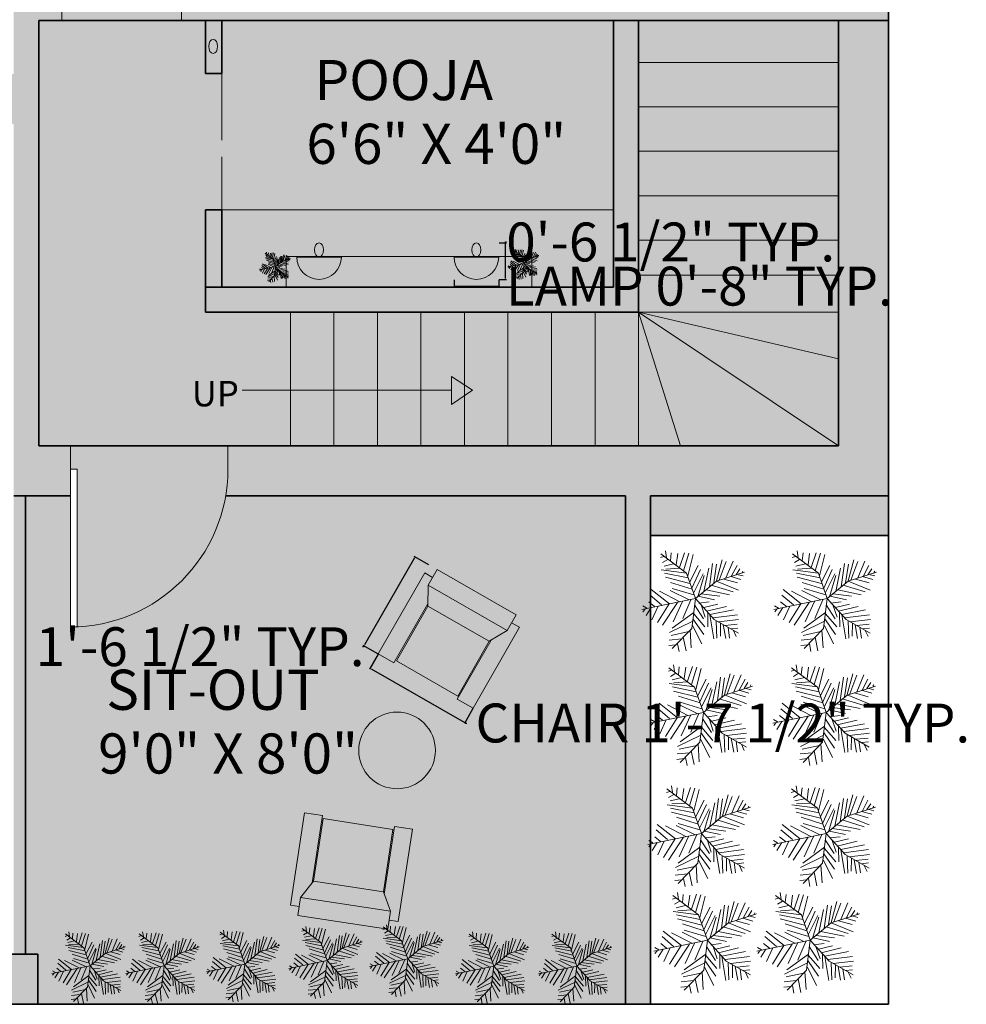
# Model space of a CAD drawing. Units: inches. Extents: x 2167 to 2589, y 1680 to 2489.
# Tile 30 of 38: x 2419 to 2589, y 1688 to 1865. Entities that reach past the tile are written whole.
import ezdxf

# ---------------------------------------------------------------- set-up
doc = ezdxf.new("R2010")
doc.units = ezdxf.units.IN
doc.header["$MEASUREMENT"] = 0
doc.linetypes.add('ACAD_ISO02W100', pattern=[15, 12, -3])
doc.layers.get('0').update_dxf_attribs({"color": 250})
for name, color, linetype, lineweight in [('A-ANNO-DIMS', 2, 'Continuous', 18), ('A-ANNO-SYMB', 7, 'Continuous', 18), ('A-AREA-IDEN', 7, 'Continuous', 18), ('A-DOOR', 4, 'Continuous', 18), ('A-FLOR-STRS', 7, 'Continuous', 18), ('A-FURN-FIXD', 34, 'Continuous', 18), ('A-FURN-PATT', 31, 'Continuous', 13), ('A-WALL-OVHD', 8, 'ACAD_ISO02W100', 18), ('A-WALL-PATT', 250, 'Continuous', 13), ('C-PROP', 7, 'Continuous', 35), ('furniture', 34, 'Continuous', 18), ('L-PLNT', 106, 'Continuous', 13), ('L-PVMT-PATT', 252, 'Continuous', 13), ('walls', 7, 'Continuous', 35)]:
    doc.layers.add(name, color=color, linetype=linetype, lineweight=lineweight)
for name, color, linetype, lineweight, true_color in [('A-FLOR-PATT', 254, 'Continuous', 13, 0xfeeab9), ('A-FLOR-STRS-PATT', 33, 'Continuous', 13, 0xcda06d), ('A-FURN-FIXD-PATT', 33, 'Continuous', 13, 0xcd8e5c)]:
    doc.layers.add(name, color=color, linetype=linetype, lineweight=lineweight, true_color=true_color)
doc.styles.get("Standard").update_dxf_attribs({"font": 'arial.ttf'})
doc.dimstyles.get("Standard").update_dxf_attribs({"dimtxt": 7, "dimasz": 0.18, "dimexe": 0.18, "dimexo": 0.0625, "dimgap": 0.09, "dimtad": 0, "dimtih": 1, "dimtoh": 1, "dimdec": 1, "dimzin": 0, "dimdsep": 46, "dimlunit": 3, "dimtxsty": 'Standard', "dimcen": 0.09, "dimadec": 0, "dimazin": 0, "dimtfac": 1, "dimtdec": 1, "dimtofl": 0, "dimtmove": 0, "dimatfit": 3, "dimfxl": 1, "dimtolj": 1, "dimtzin": 0, "dimarcsym": 0})

# ---------------------------------------------------------------- blocks, each defined once
blk = doc.blocks.new('*U2')
for p, q in [((0, 0), (0, -6)), ((40, 0), (40, -6))]:
    blk.add_line(p, q)
blk.add_lwpolyline([(0, 0), (0, 40), (1.75, 40), (1.75, 0)], close=True)
blk.add_arc((0, 0), 40, 0, 90)
blk = doc.blocks.new('*U8')
for p, q in [((-8.737, 47.138), (-17.069, 52.711)), ((-10.186, 53.64), (-13.084, 55.962)), ((0, 0), (-10.5, 57)), ((-9.099, 51.782), (-6.563, 55.962)), ((-7.288, 39.707), (-21.778, 46.673)), ((-7.65, 43.423), (-2.578, 49.46)), ((-5.839, 35.992), (4.667, 48.067)), ((-5.114, 27.632), (10.463, 46.673)), ((-3.665, 19.273), (-27.574, 35.527)), ((-5.114, 28.097), (-24.676, 40.636)), ((-2.941, 16.486), (8.652, 37.85)), ((16.259, 5.805), (23.142, 31.348)), ((22.055, 7.198), (27.489, 32.277)), ((27, 9), (48, 36)), ((27.127, 9.056), (31.112, 35.992)), ((35.096, 32.741), (37.27, 22.524)), ((38.719, 34.134), (41.979, 28.561)), ((44.153, 36.456), (45.239, 32.741)), ((-31.5, 4.5), (-52.5, 25.5)), ((-48.585, 21.131), (-49.309, 29.026)), ((-43.513, 28.561), (-42.427, 15.558)), ((-38.442, 26.239), (-34.819, 7.663)), ((-35.544, 28.097), (-24.314, 3.947)), ((-14.533, 2.09), (-30.834, 25.31)), ((-24.314, 23.917), (-2.941, 13.7)), ((-1.129, 6.734), (9.014, 26.704)), ((3.942, 1.625), (11.187, 24.381)), ((10.101, 3.483), (17.708, 26.239)), ((31.836, 30.883), (32.561, 16.486)), ((40.53, 25.775), (48.862, 24.846)), ((43.791, 29.954), (51.036, 30.883)), ((-47.498, 19.737), (-55.83, 18.344)), ((-40.615, 13.7), (-55.105, 10.913)), ((-20.691, 13.7), (-1.129, 4.876)), ((29.662, 12.307), (48.137, 6.269)), ((33.285, 16.486), (48.862, 10.913)), ((36.183, 19.737), (48.137, 17.88)), ((-33.37, 6.269), (-52.207, 5.34)), ((-28.299, 3.483), (-47.86, -5.805)), ((-21.416, 3.018), (-38.079, -8.128)), ((0, 0), (-31.5, 4.5)), ((-15.982, 2.09), (-30.11, -9.521)), ((0, 0), (-22.5, -19.5)), ((-6.563, 1.161), (-21.416, -8.128)), ((0, 0), (27, 9)), ((0, 0), (18, -22.5)), ((6.478, 1.625), (26.04, -8.592)), ((11.187, 3.483), (30.749, -5.805)), ((18.07, 5.805), (35.096, -3.483)), ((24.229, 7.663), (46.688, 1.625)), ((-6.563, -5.805), (-19.967, -9.985)), ((-9.461, -8.592), (-6.201, -23.453)), ((-4.752, -3.483), (-3.665, -14.629)), ((2.493, -3.019), (-1.491, -20.202)), ((1.769, -2.555), (24.229, -9.521)), ((5.029, -6.27), (2.131, -25.775)), ((7.565, -9.056), (32.198, -14.629)), ((-17.431, -15.094), (-42.789, -18.809)), ((-22.5, -19.5), (-37.5, -45)), ((-15.257, -12.772), (-30.11, -12.772)), ((-20.691, -18.345), (-17.793, -44.352)), ((-17.069, -15.094), (-12.721, -40.172)), ((-13.446, -11.378), (-8.737, -32.741)), ((9.014, -11.378), (3.58, -35.992)), ((14.085, -16.951), (6.478, -40.172)), ((12.274, -15.094), (36.907, -18.809)), ((16.259, -19.738), (36.183, -22.989)), ((-28.299, -29.026), (-42.789, -31.348)), ((-24.314, -21.596), (-42.427, -22.06)), ((-26.849, -26.24), (-40.253, -25.775)), ((-29.023, -30.884), (-27.936, -43.887)), ((-25.038, -23.918), (-22.865, -45.281)), ((18.07, -22.524), (8.289, -45.745)), ((20.244, -30.419), (15.897, -44.816)), ((18, -22.5), (27, -52.5)), ((18.433, -22.524), (40.53, -29.026)), ((19.157, -25.311), (38.719, -33.206)), ((-30.834, -34.135), (-42.427, -35.528)), ((-34.457, -39.708), (-40.978, -42.494)), ((-32.646, -36.921), (-31.921, -44.352)), ((22.78, -37.85), (19.519, -48.532)), ((21.331, -32.741), (39.081, -40.636)), ((22.78, -38.314), (34.372, -44.816)), ((24.591, -45.745), (23.142, -50.854)), ((24.591, -43.423), (30.749, -47.603)), ((26.764, -49.925), (28.213, -50.854))]:
    blk.add_line(p, q)
blk = doc.blocks.new('FABRIC SOFA 1S')
at = {"layer": 'furniture'}
for p, q in [((3, 18.12), (34, 18.12)), ((3, 15.12), (3, 18.12)), ((34, 12.12), (34, 18.12)), ((0, -15.12), (0, 15.12)), ((6, 15.12), (0, 15.12)), ((6, -15.12), (6, 15.12)), ((12, 11.75), (6, 15.12)), ((11.33, 12.12), (34, 12.12)), ((6, -15.12), (12, -11.75)), ((11.33, -12.12), (34, -12.12)), ((34, -12.12), (34, -18.12)), ((6, -15.12), (0, -15.12)), ((3, -18.12), (3, -15.12)), ((3, -18.12), (34, -18.12))]:
    blk.add_line(p, q, dxfattribs=at)
blk.add_lwpolyline([(12, -11.75), (12, 11.75), (33, 11.75), (33, -11.75)], close=True, dxfattribs=at)
blk = doc.blocks.new('POOJA-LAMP')
h = blk.add_hatch(color=256)
h.dxf.hatch_style = 1
edge = h.paths.add_edge_path()
edge.add_ellipse((4.02, 5.29), major_axis=(0, -1.27), ratio=0.637064, start_angle=0, end_angle=360)
blk.add_line((0, 4.02), (8.04, 4.02))
blk.add_arc((4.02, 4.02), 4.02, 180, 0)
blk.add_ellipse((4.02, 5.29), major_axis=(0, -1.27), ratio=0.637064)
blk = doc.blocks.new('*D29')
at = {"layer": 'A-ANNO-DIMS', "color": 0, "lineweight": -2, "transparency": 16777216}
for p, q in [((2483.15, 1750.65), (2481.62, 1747.99)), ((2481.87, 1748.06), (2498.61, 1738.47)), ((2500.2, 1740.88), (2498.67, 1738.22)), ((2498.76, 1738.38), (2498.92, 1738.29)), ((2498.92, 1738.29), (2499.1, 1738.29))]:
    blk.add_line(p, q, dxfattribs=at)
at = {"layer": 'A-ANNO-DIMS', "color": 0, "transparency": 16777216}
for points in [[(2481.88, 1748.09), (2481.85, 1748.04), (2481.71, 1748.15)], [(2498.62, 1738.5), (2498.59, 1738.44), (2498.76, 1738.38)]]:
    blk.add_solid(points, dxfattribs=at)
at = {"layer": 'Defpoints', "color": 0, "transparency": 16777216}
for p in [(2483.18, 1750.71), (2500.23, 1740.94), (2498.76, 1738.38)]:
    blk.add_point(p, dxfattribs=at)
at = {"layer": 'A-ANNO-DIMS', "color": 0, "transparency": 16777216, "insert": (2545.21, 1738.29), "char_height": 7, "attachment_point": 5}
blk.add_mtext('\\A1;CHAIR 1\'-7 1/2" TYP.', dxfattribs=at)
blk = doc.blocks.new('*D30')
at = {"layer": 'A-ANNO-DIMS', "color": 0, "lineweight": -2, "transparency": 16777216}
for p, q in [((2492.29, 1766.73), (2489.63, 1768.26)), ((2489.69, 1768.01), (2480.71, 1752.33)), ((2483.12, 1750.74), (2480.46, 1752.26)), ((2480.62, 1752.17), (2480.53, 1752.02)), ((2480.53, 1752.02), (2480.35, 1752.02))]:
    blk.add_line(p, q, dxfattribs=at)
at = {"layer": 'A-ANNO-DIMS', "color": 0, "transparency": 16777216}
for points in [[(2489.67, 1768.03), (2489.72, 1768), (2489.78, 1768.17)], [(2480.68, 1752.35), (2480.74, 1752.32), (2480.62, 1752.17)]]:
    blk.add_solid(points, dxfattribs=at)
at = {"layer": 'Defpoints', "color": 0, "transparency": 16777216}
for p in [(2492.34, 1766.7), (2480.62, 1752.17), (2483.18, 1750.71)]:
    blk.add_point(p, dxfattribs=at)
at = {"layer": 'A-ANNO-DIMS', "color": 0, "transparency": 16777216, "insert": (2451.1, 1752.02), "char_height": 7, "attachment_point": 5}
blk.add_mtext('\\A1;1\'-6 1/2" TYP.', dxfattribs=at)
blk = doc.blocks.new('*D47')
at = {"layer": 'A-ANNO-DIMS', "color": 0, "lineweight": -2, "transparency": 16777216}
for p, q in [((2496.82, 1818.05), (2496.82, 1816.72)), ((2504.86, 1818.05), (2504.86, 1816.72)), ((2497, 1816.9), (2504.68, 1816.9)), ((2504.86, 1816.9), (2505.04, 1816.9))]:
    blk.add_line(p, q, dxfattribs=at)
at = {"layer": 'A-ANNO-DIMS', "color": 0, "transparency": 16777216}
for points in [[(2497, 1816.93), (2497, 1816.87), (2496.82, 1816.9)], [(2504.68, 1816.93), (2504.68, 1816.87), (2504.86, 1816.9)]]:
    blk.add_solid(points, dxfattribs=at)
at = {"layer": 'Defpoints', "color": 0, "transparency": 16777216}
for p in [(2496.82, 1818.11), (2504.86, 1818.11), (2504.86, 1816.9)]:
    blk.add_point(p, dxfattribs=at)
at = {"layer": 'A-ANNO-DIMS', "color": 0, "transparency": 16777216, "insert": (2540.98, 1816.9), "char_height": 7, "attachment_point": 5}
blk.add_mtext('\\A1;LAMP 0\'-8" TYP.', dxfattribs=at)
blk = doc.blocks.new('*D48')
at = {"layer": 'A-ANNO-DIMS', "color": 0, "lineweight": -2, "transparency": 16777216}
for p, q in [((2506.06, 1824.66), (2506.06, 1824.84)), ((2506.06, 1824.84), (2506.24, 1824.84)), ((2504.92, 1824.66), (2506.24, 1824.66)), ((2506.06, 1818.29), (2506.06, 1824.48)), ((2504.92, 1818.11), (2506.24, 1818.11))]:
    blk.add_line(p, q, dxfattribs=at)
at = {"layer": 'A-ANNO-DIMS', "color": 0, "transparency": 16777216}
for points in [[(2506.03, 1824.48), (2506.09, 1824.48), (2506.06, 1824.66)], [(2506.03, 1818.29), (2506.09, 1818.29), (2506.06, 1818.11)]]:
    blk.add_solid(points, dxfattribs=at)
at = {"layer": 'Defpoints', "color": 0, "transparency": 16777216}
for p in [(2504.86, 1824.66), (2506.06, 1824.66), (2504.86, 1818.11)]:
    blk.add_point(p, dxfattribs=at)
at = {"layer": 'A-ANNO-DIMS', "color": 0, "transparency": 16777216, "insert": (2535.82, 1824.84), "char_height": 7, "attachment_point": 5}
blk.add_mtext('\\A1;0\'-6 1/2" TYP.', dxfattribs=at)

msp = doc.modelspace()

# ---------------------------------------------------------------- hatches: boundary and pattern name
at = {"layer": 'A-FLOR-PATT'}
h = msp.add_hatch(color=256, dxfattribs=at)
h.dxf.hatch_style = 1
h.paths.add_polyline_path([(2427.15, 1889.43), (2427.15, 1867.92), (2426.21, 1867.92), (2426.21, 1864.69), (2447.74, 1864.69), (2447.74, 1867.92, 0.401453)])
h = msp.add_hatch(color=256, dxfattribs=at)
h.dxf.hatch_style = 1
h.paths.add_polyline_path([(2525.55, 1864.69), (2455.04, 1864.69), (2455.04, 1855.15), (2455.04, 1830.65), (2525.55, 1830.65)])
h.paths.add_polyline_path([(2455.04, 1855.15), (2452.05, 1855.15), (2452.05, 1864.69), (2426.21, 1864.69), (2422.05, 1864.69), (2422.05, 1788.19), (2467.35, 1788.19), (2467.35, 1812.19), (2452.05, 1812.19), (2452.05, 1830.65), (2455.04, 1830.65)])
h.paths.add_polyline_path([(2419.68, 1779.19), (2417.55, 1779.19), (2417.55, 1696.69), (2419.68, 1696.69)])
at = {"layer": 'A-FLOR-STRS-PATT'}
h = msp.add_hatch(color=256, dxfattribs=at)
h.dxf.hatch_style = 1
h.paths.add_polyline_path([(2475.18, 1812.19), (2467.35, 1812.19), (2467.35, 1788.19), (2475.18, 1788.19)])
h.paths.add_polyline_path([(2483.02, 1812.19), (2475.18, 1812.19), (2475.18, 1788.19), (2483.02, 1788.19)])
h.paths.add_polyline_path([(2490.86, 1812.19), (2483.02, 1812.19), (2483.02, 1788.19), (2490.86, 1788.19)])
h.paths.add_polyline_path([(2498.7, 1812.19), (2490.86, 1812.19), (2490.86, 1788.19), (2498.7, 1788.19)])
h.paths.add_polyline_path([(2506.53, 1812.19), (2498.7, 1812.19), (2498.7, 1788.19), (2506.53, 1788.19)])
h.paths.add_polyline_path([(2514.37, 1812.19), (2506.53, 1812.19), (2506.53, 1788.19), (2514.37, 1788.19)])
h.paths.add_polyline_path([(2522.21, 1812.19), (2514.37, 1812.19), (2514.37, 1788.19), (2522.21, 1788.19)])
h.paths.add_polyline_path([(2530.05, 1812.19), (2522.21, 1812.19), (2522.21, 1788.19), (2530.05, 1788.19)])
h.paths.add_polyline_path([(2530.05, 1812.19), (2537.58, 1788.19), (2566.05, 1788.19)], flags=17)
h.paths.add_polyline_path([(2530.05, 1812.19), (2530.05, 1788.19), (2537.58, 1788.19)], flags=0)
h.paths.add_polyline_path([(2530.05, 1812.19), (2566.05, 1788.19), (2566.05, 1803.81)])
h.paths.add_polyline_path([(2566.05, 1812.19), (2530.05, 1812.19), (2566.05, 1803.81)], flags=0)
h.paths.add_polyline_path([(2566.05, 1818.88), (2530.05, 1818.88), (2530.05, 1812.19), (2566.05, 1812.19)])
h.paths.add_polyline_path([(2566.05, 1825.17), (2530.05, 1825.17), (2530.05, 1818.88), (2566.05, 1818.88)])
h.paths.add_polyline_path([(2566.05, 1833.17), (2530.05, 1833.17), (2530.05, 1825.17), (2566.05, 1825.17)])
h.paths.add_polyline_path([(2566.05, 1841.16), (2530.05, 1841.16), (2530.05, 1833.17), (2566.05, 1833.17)])
h.paths.add_polyline_path([(2566.05, 1849.15), (2530.05, 1849.15), (2530.05, 1841.16), (2566.05, 1841.16)])
h.paths.add_polyline_path([(2566.05, 1857.14), (2530.05, 1857.14), (2530.05, 1849.15), (2566.05, 1849.15)])
h.paths.add_polyline_path([(2566.05, 1864.69), (2530.05, 1864.69), (2530.05, 1857.14), (2566.05, 1857.14)])
h = msp.add_hatch(color=256, dxfattribs=at)
h.dxf.hatch_style = 1
h.paths.add_polyline_path([(2530.05, 1812.19), (2530.05, 1788.19), (2537.58, 1788.19)])
h.paths.add_polyline_path([(2566.05, 1812.19), (2530.05, 1812.19), (2566.05, 1803.81)])
at = {"layer": 'A-FURN-FIXD-PATT'}
h = msp.add_hatch(color=256, dxfattribs=at)
h.dxf.hatch_style = 1
h.paths.add_polyline_path([(2455.04, 1864.69), (2452.05, 1864.69), (2452.05, 1855.15), (2455.04, 1855.15)])
h = msp.add_hatch(color=256, dxfattribs=at)
h.dxf.hatch_style = 1
h.paths.add_polyline_path([(2525.55, 1830.65), (2455.04, 1830.65), (2455.04, 1816.69), (2466.58, 1816.69), (2466.58, 1822.24), (2510.84, 1822.24), (2510.84, 1816.69), (2525.55, 1816.69)])
h.paths.add_polyline_path([(2510.84, 1822.24), (2466.58, 1822.24), (2466.58, 1816.69), (2510.84, 1816.69)], flags=17)
at = {"layer": 'A-FURN-PATT'}
h = msp.add_hatch(color=256, dxfattribs=at)
h.dxf.hatch_style = 1
edge = h.paths.add_edge_path()
edge.add_ellipse((2453.45, 1860.03), major_axis=(0, -1.27), ratio=0.637064, start_angle=0, end_angle=360)
h = msp.add_hatch(color=256, dxfattribs=at)
h.dxf.hatch_style = 1
h.paths.add_polyline_path([(2492.14, 1763.07), (2492.11, 1759.34), (2503.16, 1753.01), (2506.37, 1754.92)])
h.paths.add_polyline_path([(2493.75, 1765.89), (2492.14, 1763.07), (2506.37, 1754.92), (2507.98, 1757.74)])
h.paths.add_polyline_path([(2492.11, 1759.75), (2492.14, 1763.07), (2492.94, 1764.48), (2491.53, 1765.29), (2483.18, 1750.71), (2486, 1749.09)])
h.paths.add_polyline_path([(2508.58, 1755.52), (2507.17, 1756.33), (2506.37, 1754.92), (2503.52, 1753.22), (2497.41, 1742.56), (2500.23, 1740.94)])
h = msp.add_hatch(color=256, dxfattribs=at)
h.dxf.hatch_style = 1
h.paths.add_polyline_path([(2503.16, 1753.01), (2492.11, 1759.34), (2486.45, 1749.46), (2497.5, 1743.13)])
h = msp.add_hatch(color=256, dxfattribs=at)
h.dxf.hatch_style = 1
h.paths.add_polyline_path([(2493.46, 1733.36, 1), (2479.66, 1733.36, 1)])
h = msp.add_hatch(color=256, dxfattribs=at)
h.dxf.hatch_style = 1
h.paths.add_polyline_path([(2485.83, 1719.16), (2473.24, 1721.09), (2471.51, 1709.84), (2484.1, 1707.9)])
h.paths.add_polyline_path([(2473.12, 1721.66), (2469.9, 1722.15), (2467.35, 1705.54), (2468.96, 1705.3), (2469.2, 1706.9), (2471.25, 1709.51)])
h.paths.add_polyline_path([(2484.1, 1707.9), (2471.51, 1709.84), (2469.2, 1706.9), (2485.41, 1704.41)])
h.paths.add_polyline_path([(2485.41, 1704.41), (2469.2, 1706.9), (2468.71, 1703.69), (2484.92, 1701.2)])
h.paths.add_polyline_path([(2489.33, 1719.17), (2486.11, 1719.66), (2484.24, 1707.52), (2485.41, 1704.41), (2485.17, 1702.8), (2486.77, 1702.56)])
at = {"layer": 'A-WALL-PATT'}
h = msp.add_hatch(color=256, dxfattribs=at)
h.dxf.hatch_style = 1
h.paths.add_polyline_path([(2575.05, 2029.69), (2422.05, 2029.69), (2422.05, 2161.69), (2427.02, 2161.69), (2427.02, 2161.94), (2427.02, 2166.19), (2417.55, 2166.19), (2417.55, 2025.19), (2575.05, 2025.19)])
h.paths.add_polyline_path([(2575.05, 2166.19), (2503.01, 2166.19), (2503.01, 2161.69), (2575.05, 2161.69)], flags=17)
h.paths.add_polyline_path([(2575.05, 2161.69), (2566.05, 2161.69), (2566.05, 2029.69), (2575.05, 2029.69)], flags=17)
h.paths.add_polyline_path([(2575.05, 2025.19), (2566.05, 2025.19), (2566.05, 1869.19), (2575.05, 1869.19)])
h.paths.add_polyline_path([(2575.05, 1869.19), (2566.05, 1869.19), (2447.7, 1869.19, -0.014764), (2447.74, 1867.92), (2447.74, 1864.69), (2575.05, 1864.69)])
h.paths.add_polyline_path([(2530.05, 1864.69), (2525.55, 1864.69), (2525.55, 1816.69), (2452.05, 1816.69), (2452.05, 1812.19), (2530.05, 1812.19)])
h.paths.add_polyline_path([(2455.04, 1830.65), (2452.05, 1830.65), (2452.05, 1816.69), (2455.04, 1816.69)], flags=17)
h.paths.add_polyline_path([(2575.05, 1864.69), (2566.05, 1864.69), (2566.05, 1788.19), (2456.1, 1788.19), (2456.1, 1783.94, -0.042065), (2455.7, 1779.19), (2527.68, 1779.19), (2527.68, 1687.69), (2532.18, 1687.69), (2532.18, 1779.19), (2575.05, 1779.19)])
h.paths.add_polyline_path([(2421.87, 1696.69), (2416.11, 1696.69), (2416.11, 1687.69), (2421.87, 1687.69)])
h.paths.add_polyline_path([(2375.61, 1696.69), (2369.84, 1696.69), (2369.84, 1687.69), (2375.61, 1687.69)])
h.paths.add_polyline_path([(2425.05, 2245.69), (2420.55, 2245.69), (2420.55, 2226.19), (2432.29, 2226.19), (2432.29, 2229.42), (2432.29, 2230.69), (2425.05, 2230.69)])
h.paths.add_polyline_path([(2224.05, 2151.19), (2318.55, 2151.19), (2318.55, 2177.3), (2314.78, 2177.3, -0.007324), (2314.05, 2177.32), (2314.05, 2155.69), (2224.05, 2155.69), (2224.05, 2157.46), (2215.05, 2157.46), (2215.05, 2103.59), (2218.97, 2103.59), (2224.05, 2103.59)])
h = msp.add_hatch(color=256, dxfattribs=at)
h.dxf.hatch_style = 1
h.paths.add_polyline_path([(2274.74, 1855.04), (2224.05, 1855.04), (2224.05, 2003.12), (2215.05, 2003.12), (2215.05, 1846.04), (2274.74, 1846.04)])
h.paths.add_polyline_path([(2354.89, 1855.04), (2330.89, 1855.04), (2330.89, 1846.04), (2354.77, 1846.04), (2354.77, 1852.04, -0.01877)])
h.paths.add_polyline_path([(2422.05, 1864.69), (2426.21, 1864.69), (2426.21, 1867.92), (2426.21, 1869.19), (2422.05, 1869.19), (2422.05, 1916.24), (2417.55, 1916.24), (2417.55, 1855.04), (2394.77, 1855.04), (2394.77, 1852.04), (2394.77, 1846.04), (2417.55, 1846.04), (2417.55, 1779.19), (2427.74, 1779.19), (2427.74, 1783.94), (2427.74, 1788.19), (2422.05, 1788.19)])
at = {"layer": 'L-PVMT-PATT'}
h = msp.add_hatch(color=256, dxfattribs=at)
h.dxf.hatch_style = 1
h.paths.add_polyline_path([(2527.68, 1779.19), (2455.7, 1779.19, -0.35342), (2428.98, 1755.61), (2428.98, 1755.58), (2427.74, 1755.58), (2427.74, 1779.19), (2419.68, 1779.19), (2419.68, 1696.69), (2421.87, 1696.69), (2421.87, 1687.69), (2527.68, 1687.69)])
h.paths.add_polyline_path([(2493.46, 1733.36, -1), (2479.66, 1733.36, -1)], flags=16)
h.paths.add_polyline_path([(2483.18, 1750.71), (2491.53, 1765.29), (2492.94, 1764.48), (2493.75, 1765.89), (2507.98, 1757.74), (2507.17, 1756.33), (2508.58, 1755.52), (2500.23, 1740.94), (2497.41, 1742.56), (2497.68, 1743.03), (2486.27, 1749.56), (2486, 1749.09)], flags=16)
h.paths.add_polyline_path([(2469.9, 1722.15), (2473.12, 1721.66), (2473.03, 1721.12), (2486.03, 1719.13), (2486.11, 1719.66), (2489.33, 1719.17), (2486.77, 1702.56), (2485.17, 1702.8), (2484.92, 1701.2), (2468.71, 1703.69), (2468.96, 1705.3), (2467.35, 1705.54)], flags=16)
h.paths.add_polyline_path([(2456.1, 1783.94), (2456.1, 1788.19), (2427.74, 1788.19), (2427.74, 1783.94), (2428.98, 1783.94), (2428.98, 1755.61, 0.401453)])
h = msp.add_hatch(color=256, dxfattribs=at)
h.dxf.hatch_style = 1
h.paths.add_polyline_path([(2575.05, 1779.19), (2532.18, 1779.19), (2532.18, 1772.02), (2575.05, 1772.02)])

# ---------------------------------------------------------------- linework, layer by layer
at = {"layer": 'A-ANNO-SYMB'}
for p, q in [((2500.16, 1798.2), (2496.35, 1800.63)), ((2496.35, 1800.63), (2496.35, 1798.2)), ((2458.68, 1798.2), (2496.35, 1798.2)), ((2496.35, 1798.2), (2496.35, 1795.61)), ((2496.35, 1795.61), (2500.16, 1798.2))]:
    msp.add_line(p, q, dxfattribs=at)
at = {"layer": 'A-FLOR-STRS'}
for p, q in [((2530.05, 1857.14), (2566.05, 1857.14)), ((2530.05, 1849.15), (2566.05, 1849.15)), ((2530.05, 1841.16), (2566.05, 1841.16)), ((2530.05, 1833.17), (2566.05, 1833.17)), ((2530.05, 1825.17), (2566.05, 1825.17)), ((2530.05, 1818.88), (2566.05, 1818.88)), ((2467.35, 1812.19), (2467.35, 1788.19)), ((2475.18, 1812.19), (2475.18, 1788.19)), ((2483.02, 1812.19), (2483.02, 1788.19)), ((2490.86, 1812.19), (2490.86, 1788.19)), ((2498.7, 1812.19), (2498.7, 1788.19)), ((2506.53, 1812.19), (2506.53, 1788.19)), ((2514.37, 1812.19), (2514.37, 1788.19)), ((2522.21, 1812.19), (2522.21, 1788.19)), ((2530.05, 1812.19), (2566.05, 1812.19)), ((2530.05, 1812.19), (2530.05, 1788.19)), ((2530.05, 1812.19), (2566.05, 1788.19)), ((2530.05, 1812.19), (2537.58, 1788.19)), ((2530.05, 1812.19), (2566.05, 1803.81))]:
    msp.add_line(p, q, dxfattribs=at)
at = {"layer": 'A-FURN-FIXD'}
for p, q in [((2455.04, 1830.65), (2525.55, 1830.65)), ((2466.58, 1816.69), (2466.58, 1822.24)), ((2466.58, 1822.24), (2510.84, 1822.24)), ((2510.84, 1822.24), (2510.84, 1816.69))]:
    msp.add_line(p, q, dxfattribs=at)
at = {"layer": 'A-WALL-OVHD'}
msp.add_line((2455.04, 1855.15), (2455.04, 1830.65), dxfattribs=at)
at = {"layer": 'C-PROP'}
for p, q in [((2575.05, 2407.69), (2575.05, 1687.69)), ((2575.05, 1687.69), (2215.05, 1687.69))]:
    msp.add_line(p, q, dxfattribs=at)
at = {"layer": 'furniture'}
msp.add_circle((2486.56, 1733.36), 6.9, dxfattribs=at)
msp.add_ellipse((2453.45, 1860.03), major_axis=(0, -1.27), ratio=0.637064, dxfattribs=at)
at = {"layer": 'walls'}
for p, q in [((2422.05, 1864.69), (2426.21, 1864.69)), ((2422.05, 1864.69), (2422.05, 1788.19)), ((2426.21, 1864.69), (2575.05, 1864.69)), ((2452.05, 1864.69), (2452.05, 1855.15)), ((2455.04, 1864.69), (2455.04, 1855.15)), ((2525.55, 1864.69), (2525.55, 1816.69)), ((2530.05, 1864.69), (2530.05, 1812.19)), ((2566.05, 1864.69), (2566.05, 1788.19)), ((2452.05, 1855.15), (2455.04, 1855.15)), ((2452.05, 1830.65), (2455.04, 1830.65)), ((2452.05, 1830.65), (2452.05, 1812.19)), ((2455.04, 1830.65), (2455.04, 1816.69)), ((2452.05, 1816.69), (2525.55, 1816.69)), ((2452.05, 1812.19), (2530.05, 1812.19)), ((2566.05, 1788.19), (2422.05, 1788.19)), ((2427.74, 1779.19), (2417.55, 1779.19)), ((2419.68, 1779.19), (2419.68, 1696.69)), ((2527.68, 1779.19), (2455.7, 1779.19)), ((2527.68, 1779.19), (2527.68, 1687.69)), ((2532.18, 1779.19), (2532.18, 1687.69)), ((2575.05, 1779.19), (2532.18, 1779.19)), ((2532.18, 1772.02), (2575.05, 1772.02)), ((2421.87, 1696.69), (2416.11, 1696.69)), ((2421.87, 1696.69), (2421.87, 1687.69))]:
    msp.add_line(p, q, dxfattribs=at)

# ---------------------------------------------------------------- block references
at = {"layer": 'A-DOOR', "xscale": 0.5382298898187942, "yscale": 0.5382298898187942, "zscale": 0.5382298898187942}
msp.add_blockref('*U2', (2426.21, 1867.92), dxfattribs=at)
at = {"layer": 'A-DOOR', "xscale": -0.7089553820317277, "yscale": 0.7089553820317277, "zscale": 0.7089553820317277, "rotation": 180}
msp.add_blockref('*U2', (2427.74, 1783.94), dxfattribs=at)
at = {"layer": 'furniture'}
for p in [(2468.49, 1818.11), (2496.82, 1818.11)]:
    msp.add_blockref('POOJA-LAMP', p, dxfattribs=at)
at = {"layer": 'furniture', "yscale": 0.5421468747490584, "zscale": 0.5421468747490584}
for p, xscale, rotation in [((2500.87, 1761.82), 0.5421468747490584, 240.1897580650286), ((2476.81, 1702.44), -0.5421468747490583, 261.2590712397156)]:
    msp.add_blockref('FABRIC SOFA 1S', p, dxfattribs=dict(at, xscale=xscale, rotation=rotation))
at = {"layer": 'L-PLNT', "rotation": 90.98387132377816}
for p, xscale, yscale, zscale in [((2464.7, 1820.41), 0.0510892351028333, 0.0510892351028333, 0.0510892351028333), ((2509.43, 1820.96), 0.0510892351028333, 0.0510892351028333, 0.0510892351028333), ((2540.28, 1760.67), 0.1698531738429223, 0.1698531738429223, 0.1698531738429223), ((2564.01, 1760.67), 0.1698531738429223, 0.1698531738429223, 0.1698531738429223), ((2541.72, 1740.2), 0.1698531738429223, 0.1698531738429223, 0.1698531738429223), ((2563.83, 1740.2), 0.1698531738429223, 0.1698531738429223, 0.1698531738429223), ((2541.36, 1718.41), 0.1698531738429223, 0.1698531738429223, 0.1698531738429223), ((2563.83, 1718.41), 0.1698531738429223, 0.1698531738429223, 0.1698531738429223), ((2542.44, 1699.2), 0.1698531738429223, 0.1698531738429223, 0.1698531738429223), ((2560.95, 1699.2), 0.1698531738429223, 0.1698531738429223, 0.1698531738429223), ((2431.31, 1694.61), 0.1214066606707073, 0.1214066606707073, 0.1214066606707073), ((2444.61, 1694.61), 0.1214066606707073, 0.1214066606707073, 0.1214066606707073), ((2459.16, 1694.91), 0.1214066606707073, 0.1214066606707073, 0.1214066606707073), ((2473.96, 1695.54), 0.1214066606707073, 0.1214066606707073, 0.1214066606707073), ((2488.52, 1695.85), 0.1214066606707073, 0.1214066606707073, 0.1214066606707073), ((2503.99, 1694.57), 0.1214066606707073, 0.1214066606707073, 0.1214066606707073), ((2518.92, 1694.57), 0.1214066606707073, 0.1214066606707073, 0.1214066606707073)]:
    msp.add_blockref('*U8', p, dxfattribs=dict(at, xscale=xscale, yscale=yscale, zscale=zscale))

# ---------------------------------------------------------------- texts
at = {"layer": 'A-ANNO-SYMB'}
msp.add_text('UP', height=4.586, dxfattribs=at).set_placement((2449.6, 1795.26))
at = {"layer": 'A-AREA-IDEN'}
for s, height, p in [('POOJA', 7.227, (2471.71, 1850.36)), ('6\'6" X 4\'0"', 7.2272, (2470.23, 1838.89)), ('SIT-OUT', 7.227, (2434.21, 1740.66)), ('9\'0" X 8\'0"', 7.2272, (2432.74, 1729.19))]:
    msp.add_text(s, height=height, dxfattribs=at).set_placement(p)

# ---------------------------------------------------------------- dimensions: what is measured, and where the dimension line sits
at = {"layer": 'A-ANNO-DIMS'}
for base, p1, p2, angle, text, picture, middle in [((2506.0622, 1824.664), (2504.8568, 1818.1084), (2504.8568, 1824.664), 90, '<> TYP.', '*D48', (2535.822, 1824.844)), ((2480.62, 1752.17), (2492.34, 1766.7), (2483.18, 1750.71), 240.1898, '<> TYP.', '*D30', (2451.1, 1752.02)), ((2498.76, 1738.38), (2483.18, 1750.71), (2500.23, 1740.94), 330.1898, 'CHAIR <> TYP.', '*D29', (2545.21, 1738.29))]:
    dim = msp.add_linear_dim(base=base, p1=p1, p2=p2, angle=angle, text=text, dimstyle='Standard', override={"dimdec": 1, "dimlfac": 1, "dimrnd": 0, "dimzin": 1, "dimdsep": 46, "dimlunit": 4, "dimfrac": 2}, dxfattribs=at)
    dim.commit()
    dim.dimension.update_dxf_attribs({"geometry": picture, "text_midpoint": middle})
dim = msp.add_linear_dim(base=(2504.86, 1816.9), p1=(2496.82, 1818.11), p2=(2504.86, 1818.11), text='LAMP <> TYP.', dimstyle='Standard', override={"dimdec": 1, "dimlfac": 1, "dimrnd": 0, "dimzin": 1, "dimdsep": 46, "dimlunit": 4, "dimfrac": 2}, dxfattribs=at)
dim.commit()
dim.dimension.update_dxf_attribs({"geometry": '*D47', "text_midpoint": (2540.98, 1816.9)})

doc.saveas('drawing.dxf')
